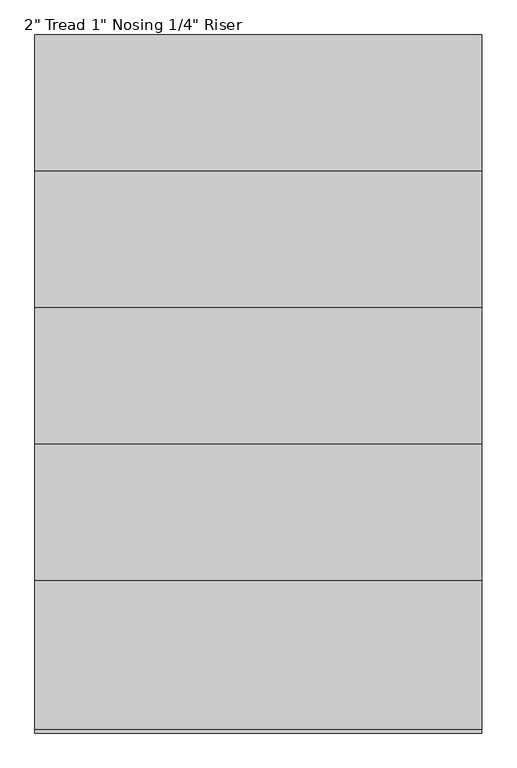
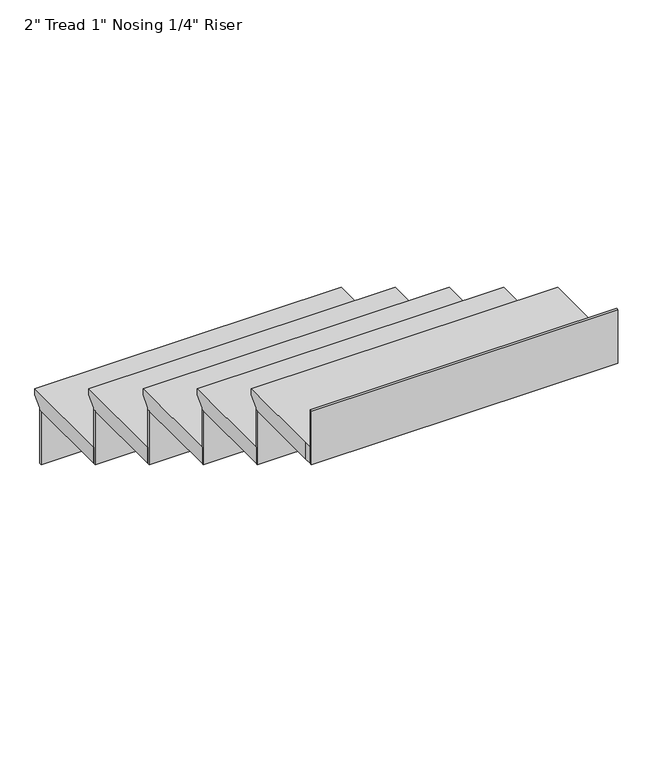
"""IFC4 building model written with IfcOpenShell, lengths in millimetres: stair flight geometry."""

from ifc_helpers import new_model, si_unit, origin, place, context, project, spatial, faceted_brep, source, transform, mapped, element, save


def stair_flight_4bd381d9(model_context):
    return source(origin(), model_context, "Body", "Brep", [
        faceted_brep([(-803.1608498, 3514.5115866, 4383.6166667), (-803.1608498, 3514.5115866, 4402.6666667), (111.2391502, 3514.5115866, 4402.6666667), (111.2391502, 3514.5115866, 4383.6166667), (-803.1608498, 3489.1115866, 4358.2166667), (111.2391502, 3489.1115866, 4358.2166667), (-803.1608498, 3209.7115866, 4402.6666667), (111.2391502, 3209.7115866, 4402.6666667), (111.2391502, 3489.1115866, 4351.8666667), (111.2391502, 3209.7115866, 4351.8666667), (-803.1608498, 3209.7115866, 4351.8666667), (-803.1608498, 3489.1115866, 4351.8666667)], [[[0, 1, 2, 3]], [[4, 0, 3, 5]], [[2, 1, 6, 7]], [[8, 9, 10, 11]], [[2, 7, 9, 8, 5, 3]], [[8, 11, 4, 5]], [[6, 1, 0, 4, 11, 10]], [[7, 6, 10, 9]]]),
        faceted_brep([(-803.1608498, 3489.1115866, 4351.8666667), (-803.1608498, 3489.1115866, 4182.5333333), (-803.1608498, 3482.7615866, 4182.5333333), (-803.1608498, 3482.7615866, 4351.8666667), (111.2391502, 3489.1115866, 4351.8666667), (111.2391502, 3482.7615866, 4351.8666667), (111.2391502, 3482.7615866, 4182.5333333), (111.2391502, 3489.1115866, 4182.5333333)], [[[0, 1, 2, 3]], [[4, 5, 6, 7]], [[1, 0, 4, 7]], [[2, 1, 7, 6]], [[3, 2, 6, 5]], [[0, 3, 5, 4]]]),
        faceted_brep([(-803.1608498, 3209.7115866, 4521.2), (-803.1608498, 3209.7115866, 4351.8666667), (-803.1608498, 3203.3615866, 4351.8666667), (-803.1608498, 3203.3615866, 4521.2), (111.2391502, 3209.7115866, 4521.2), (111.2391502, 3203.3615866, 4521.2), (111.2391502, 3203.3615866, 4351.8666667), (111.2391502, 3209.7115866, 4351.8666667)], [[[0, 1, 2, 3]], [[4, 5, 6, 7]], [[1, 0, 4, 7]], [[2, 1, 7, 6]], [[3, 2, 6, 5]], [[0, 3, 5, 4]]]),
        faceted_brep([(111.2391502, 3235.1115866, 4572.0), (-803.1608498, 3235.1115866, 4572.0), (-803.1608498, 2930.3115866, 4572.0), (111.2391502, 2930.3115866, 4572.0), (111.2391502, 3209.7115866, 4521.2), (111.2391502, 2930.3115866, 4521.2), (-803.1608498, 2930.3115866, 4521.2), (-803.1608498, 3209.7115866, 4521.2), (111.2391502, 3209.7115866, 4527.55), (111.2391502, 3235.1115866, 4552.95), (-803.1608498, 3209.7115866, 4527.55), (-803.1608498, 3235.1115866, 4552.95)], [[[0, 1, 2, 3]], [[4, 5, 6, 7]], [[0, 3, 5, 4, 8, 9]], [[4, 7, 10, 8]], [[2, 1, 11, 10, 7, 6]], [[3, 2, 6, 5]], [[11, 1, 0, 9]], [[10, 11, 9, 8]]]),
        faceted_brep([(-803.1608498, 2930.3115866, 4690.5333333), (-803.1608498, 2930.3115866, 4521.2), (-803.1608498, 2923.9615866, 4521.2), (-803.1608498, 2923.9615866, 4690.5333333), (111.2391502, 2930.3115866, 4690.5333333), (111.2391502, 2923.9615866, 4690.5333333), (111.2391502, 2923.9615866, 4521.2), (111.2391502, 2930.3115866, 4521.2)], [[[0, 1, 2, 3]], [[4, 5, 6, 7]], [[1, 0, 4, 7]], [[2, 1, 7, 6]], [[3, 2, 6, 5]], [[0, 3, 5, 4]]]),
        faceted_brep([(111.2391502, 2955.7115866, 4741.3333333), (-803.1608498, 2955.7115866, 4741.3333333), (-803.1608498, 2650.9115866, 4741.3333333), (111.2391502, 2650.9115866, 4741.3333333), (111.2391502, 2930.3115866, 4690.5333333), (111.2391502, 2650.9115866, 4690.5333333), (-803.1608498, 2650.9115866, 4690.5333333), (-803.1608498, 2930.3115866, 4690.5333333), (111.2391502, 2930.3115866, 4696.8833333), (111.2391502, 2955.7115866, 4722.2833333), (-803.1608498, 2930.3115866, 4696.8833333), (-803.1608498, 2955.7115866, 4722.2833333)], [[[0, 1, 2, 3]], [[4, 5, 6, 7]], [[0, 3, 5, 4, 8, 9]], [[4, 7, 10, 8]], [[2, 1, 11, 10, 7, 6]], [[3, 2, 6, 5]], [[11, 1, 0, 9]], [[10, 11, 9, 8]]]),
        faceted_brep([(-803.1608498, 2650.9115866, 4859.8666667), (-803.1608498, 2650.9115866, 4690.5333333), (-803.1608498, 2644.5615866, 4690.5333333), (-803.1608498, 2644.5615866, 4859.8666667), (111.2391502, 2650.9115866, 4859.8666667), (111.2391502, 2644.5615866, 4859.8666667), (111.2391502, 2644.5615866, 4690.5333333), (111.2391502, 2650.9115866, 4690.5333333)], [[[0, 1, 2, 3]], [[4, 5, 6, 7]], [[1, 0, 4, 7]], [[2, 1, 7, 6]], [[3, 2, 6, 5]], [[0, 3, 5, 4]]]),
        faceted_brep([(111.2391502, 2676.3115866, 4910.6666667), (-803.1608498, 2676.3115866, 4910.6666667), (-803.1608498, 2371.5115866, 4910.6666667), (111.2391502, 2371.5115866, 4910.6666667), (111.2391502, 2650.9115866, 4859.8666667), (111.2391502, 2371.5115866, 4859.8666667), (-803.1608498, 2371.5115866, 4859.8666667), (-803.1608498, 2650.9115866, 4859.8666667), (111.2391502, 2650.9115866, 4866.2166667), (111.2391502, 2676.3115866, 4891.6166667), (-803.1608498, 2650.9115866, 4866.2166667), (-803.1608498, 2676.3115866, 4891.6166667)], [[[0, 1, 2, 3]], [[4, 5, 6, 7]], [[0, 3, 5, 4, 8, 9]], [[4, 7, 10, 8]], [[2, 1, 11, 10, 7, 6]], [[3, 2, 6, 5]], [[11, 1, 0, 9]], [[10, 11, 9, 8]]]),
        faceted_brep([(-803.1608498, 2092.1115866, 5198.5333333), (-803.1608498, 2092.1115866, 5029.2), (-803.1608498, 2085.7615866, 5029.2), (-803.1608498, 2085.7615866, 5198.5333333), (111.2391502, 2092.1115866, 5198.5333333), (111.2391502, 2085.7615866, 5198.5333333), (111.2391502, 2085.7615866, 5029.2), (111.2391502, 2092.1115866, 5029.2)], [[[0, 1, 2, 3]], [[4, 5, 6, 7]], [[1, 0, 4, 7]], [[2, 1, 7, 6]], [[3, 2, 6, 5]], [[0, 3, 5, 4]]]),
        faceted_brep([(-803.1608498, 2371.5115866, 5029.2), (-803.1608498, 2371.5115866, 4859.8666667), (-803.1608498, 2365.1615866, 4859.8666667), (-803.1608498, 2365.1615866, 5029.2), (111.2391502, 2371.5115866, 5029.2), (111.2391502, 2365.1615866, 5029.2), (111.2391502, 2365.1615866, 4859.8666667), (111.2391502, 2371.5115866, 4859.8666667)], [[[0, 1, 2, 3]], [[4, 5, 6, 7]], [[1, 0, 4, 7]], [[2, 1, 7, 6]], [[3, 2, 6, 5]], [[0, 3, 5, 4]]]),
        faceted_brep([(111.2391502, 2092.1115866, 5080.0), (111.2391502, 2117.5115866, 5080.0), (111.2391502, 2396.9115866, 5080.0), (-803.1608498, 2396.9115866, 5080.0), (-803.1608498, 2117.5115866, 5080.0), (-803.1608498, 2092.1115866, 5080.0), (111.2391502, 2117.5115866, 5029.2), (111.2391502, 2092.1115866, 5029.2), (-803.1608498, 2092.1115866, 5029.2), (-803.1608498, 2117.5115866, 5029.2), (-803.1608498, 2371.5115866, 5029.2), (111.2391502, 2371.5115866, 5029.2), (111.2391502, 2371.5115866, 5035.55), (111.2391502, 2396.9115866, 5060.95), (-803.1608498, 2371.5115866, 5035.55), (-803.1608498, 2396.9115866, 5060.95)], [[[0, 1, 2, 3, 4, 5]], [[6, 7, 8, 9, 10, 11]], [[1, 0, 7, 6]], [[2, 1, 6, 11, 12, 13]], [[11, 10, 14, 12]], [[4, 3, 15, 14, 10, 9]], [[5, 4, 9, 8]], [[0, 5, 8, 7]], [[15, 3, 2, 13]], [[14, 15, 13, 12]]]),
    ])


if __name__ == "__main__":
    model = new_model("IFC4")
    model_context = context("Model", 3, world=origin())
    ifc_project = project(units=[si_unit("LENGTHUNIT", "METRE", prefix="MILLI")], contexts=[model_context])
    site = spatial("IfcSite", under=ifc_project)
    building = spatial("IfcBuilding", under=site)
    placement = place(None, origin())
    stair_flight_shape = stair_flight_4bd381d9(model_context)
    element("IfcStairFlight", 1, ObjectType="2\" Tread 1\" Nosing 1/4\" Riser", at=placement, inside=building, context=model_context, shape_type="MappedRepresentation", body=[
        mapped(stair_flight_shape, transform((0.0, 0.0, 0.0), x_axis=(1.0, 0.0, 0.0), y_axis=(0.0, 1.0, 0.0), z_axis=(0.0, 0.0, 1.0))),
    ])
    save(model, "model.ifc")
